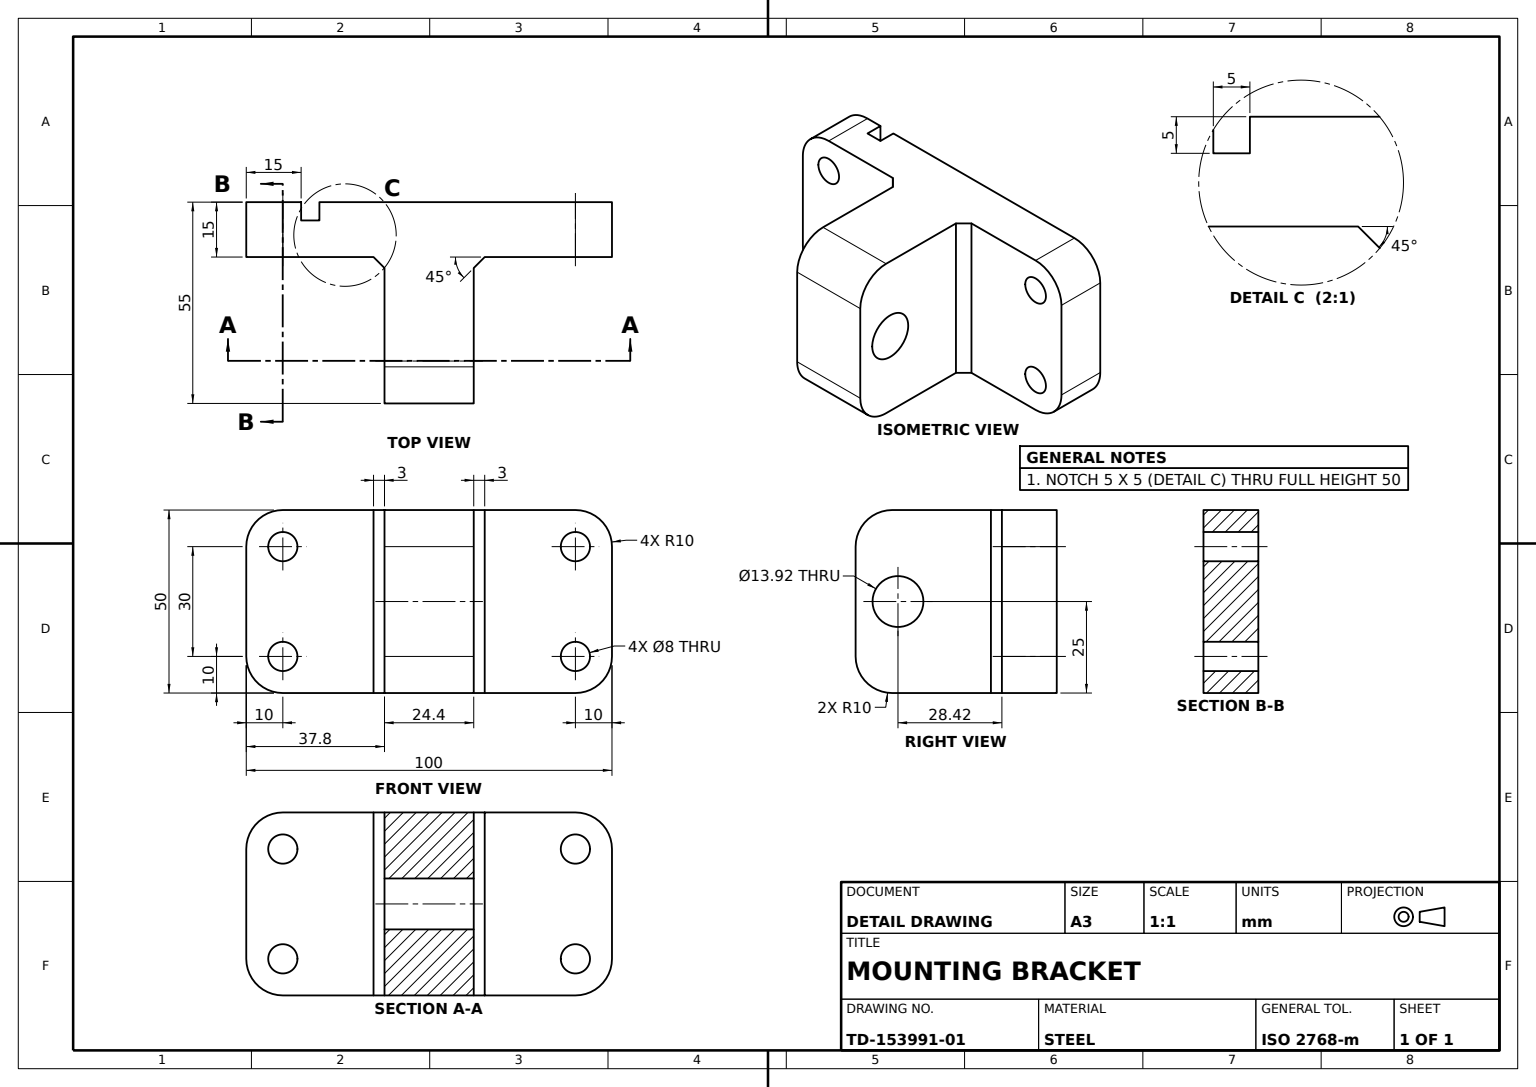
from build123d import *

# Parameters (mm, degrees)
BASE_PLATE_DEPTH              = 15
KNUCKLE_BLOCK_DEPTH           = 100
KNUCKLE_RELIEF_CUT_A_DEPTH    = 37.8
KNUCKLE_START                 = -37.8
KNUCKLE_RELIEF_CUT_B_DEPTH    = 37.8
PLATE_MOUNTING_HOLES_SKETCH_W = 5
PLATE_MOUNTING_HOLES_SKETCH_H = 5
PLATE_MOUNTING_HOLES_DEPTH    = 50
HINGE_PIN_HOLE_SKETCH_R       = 6.957950298
HINGE_PIN_HOLE_DEPTH          = 50
UPPER_MOUNTING_HOLES_SKETCH_R = 4
UPPER_MOUNTING_HOLES_DEPTH    = 50
KNUCKLE_CHAMFER_A_3X45_SIZE   = 3
KNUCKLE_CHAMFER_B_3X45_SIZE   = 3


with BuildPart() as part:
    # Base Plate Sketch → Base Plate (new body)
    with BuildSketch(Plane.XY):
        with BuildLine():
            Line((10, 0), (90, 0))
            ThreePointArc((90, 0), (97.071067812, 2.928932188), (100, 10))
            Line((100, 10), (100, 40))
            ThreePointArc((100, 40), (97.071067812, 47.071067812), (90, 50))
            Line((90, 50), (10, 50))
            ThreePointArc((10, 50), (2.928932188, 47.071067812), (0, 40))
            Line((0, 40), (0, 10))
            ThreePointArc((0, 10), (2.928932188, 2.928932188), (10, 0))
        make_face()
    extrude(amount=BASE_PLATE_DEPTH)

    # Knuckle Block Sketch → Knuckle Block (add)
    with BuildSketch(Plane(origin=(100, 0, 0), x_dir=(0, 0, -1), z_dir=(1, 0, 0))):
        with BuildLine():
            Line((-15, 50), (-45, 50))
            ThreePointArc((-45, 50), (-52.071067812, 47.071067812), (-55, 40))
            Line((-55, 40), (-55, 10))
            ThreePointArc((-55, 10), (-52.071067812, 2.928932188), (-45, 0))
            Line((-45, 0), (-15, 0))
            Line((-15, 0), (-15, 50))
        make_face()
    extrude(amount=-KNUCKLE_BLOCK_DEPTH)

    # Knuckle Relief Cut A Sketch → Knuckle Relief Cut A (cut)
    with BuildSketch(Plane(origin=(100, 0, 0), x_dir=(0, 0, -1), z_dir=(1, 0, 0))):
        with BuildLine():
            Line((-15, 40), (-15, 50))
            Line((-15, 50), (-45, 50))
            ThreePointArc((-45, 50), (-52.071067812, 47.071067812), (-55, 40))
            Line((-55, 40), (-55, 10))
            ThreePointArc((-55, 10), (-52.071067812, 2.928932188), (-45, 0))
            Line((-45, 0), (-15, 0))
            Line((-15, 0), (-15, 40))
        make_face()
    extrude(amount=-KNUCKLE_RELIEF_CUT_A_DEPTH, mode=Mode.SUBTRACT)

    # Knuckle Relief Cut B Sketch → Knuckle Relief Cut B (cut)
    with BuildSketch(Plane.ZY.offset(KNUCKLE_START)):
        with BuildLine():
            Line((15, 50), (45, 50))
            ThreePointArc((45, 50), (52.071067812, 47.071067812), (55, 40))
            Line((55, 40), (55, 10))
            ThreePointArc((55, 10), (52.071067812, 2.928932188), (45, 0))
            Line((45, 0), (15, 0))
            Line((15, 0), (15, 50))
        make_face()
    extrude(amount=KNUCKLE_RELIEF_CUT_B_DEPTH, mode=Mode.SUBTRACT)

    # Plate Mounting Holes Sketch → Plate Mounting Holes (cut)
    with BuildSketch(Plane.XZ):
        with Locations((17.5, 2.5)):
            Rectangle(PLATE_MOUNTING_HOLES_SKETCH_W, PLATE_MOUNTING_HOLES_SKETCH_H)
    extrude(amount=-PLATE_MOUNTING_HOLES_DEPTH, mode=Mode.SUBTRACT)

    # Hinge Pin Hole Sketch → Hinge Pin Hole (cut)
    with BuildSketch(Plane(origin=(62.2, 0, 0), x_dir=(0, 0, -1), z_dir=(1, 0, 0))):
        with Locations((-43.415970908, 25)):
            Circle(HINGE_PIN_HOLE_SKETCH_R)
    extrude(amount=-HINGE_PIN_HOLE_DEPTH, mode=Mode.SUBTRACT)

    # Upper Mounting Holes Sketch → Upper Mounting Holes (cut)
    with BuildSketch(Plane.XY.offset(15)):
        with Locations((90, 40)):
            Circle(UPPER_MOUNTING_HOLES_SKETCH_R)
        with Locations((90, 10)):
            Circle(UPPER_MOUNTING_HOLES_SKETCH_R)
        with Locations((10, 40)):
            Circle(UPPER_MOUNTING_HOLES_SKETCH_R)
        with Locations((10, 10)):
            Circle(UPPER_MOUNTING_HOLES_SKETCH_R)
    extrude(amount=-UPPER_MOUNTING_HOLES_DEPTH, mode=Mode.SUBTRACT)

    # Knuckle Chamfer A 3x45
    knuckle_chamfer_a_3x45_edges = [part.edges().sort_by_distance(p)[0] for p in [
        (62.2, 25, 15),
    ]]
    chamfer(knuckle_chamfer_a_3x45_edges, length=KNUCKLE_CHAMFER_A_3X45_SIZE)

    # Knuckle Chamfer B 3x45
    knuckle_chamfer_b_3x45_edges = [part.edges().sort_by_distance(p)[0] for p in [
        (37.8, 25, 15),
    ]]
    chamfer(knuckle_chamfer_b_3x45_edges, length=KNUCKLE_CHAMFER_B_3X45_SIZE)


solid = part.part
